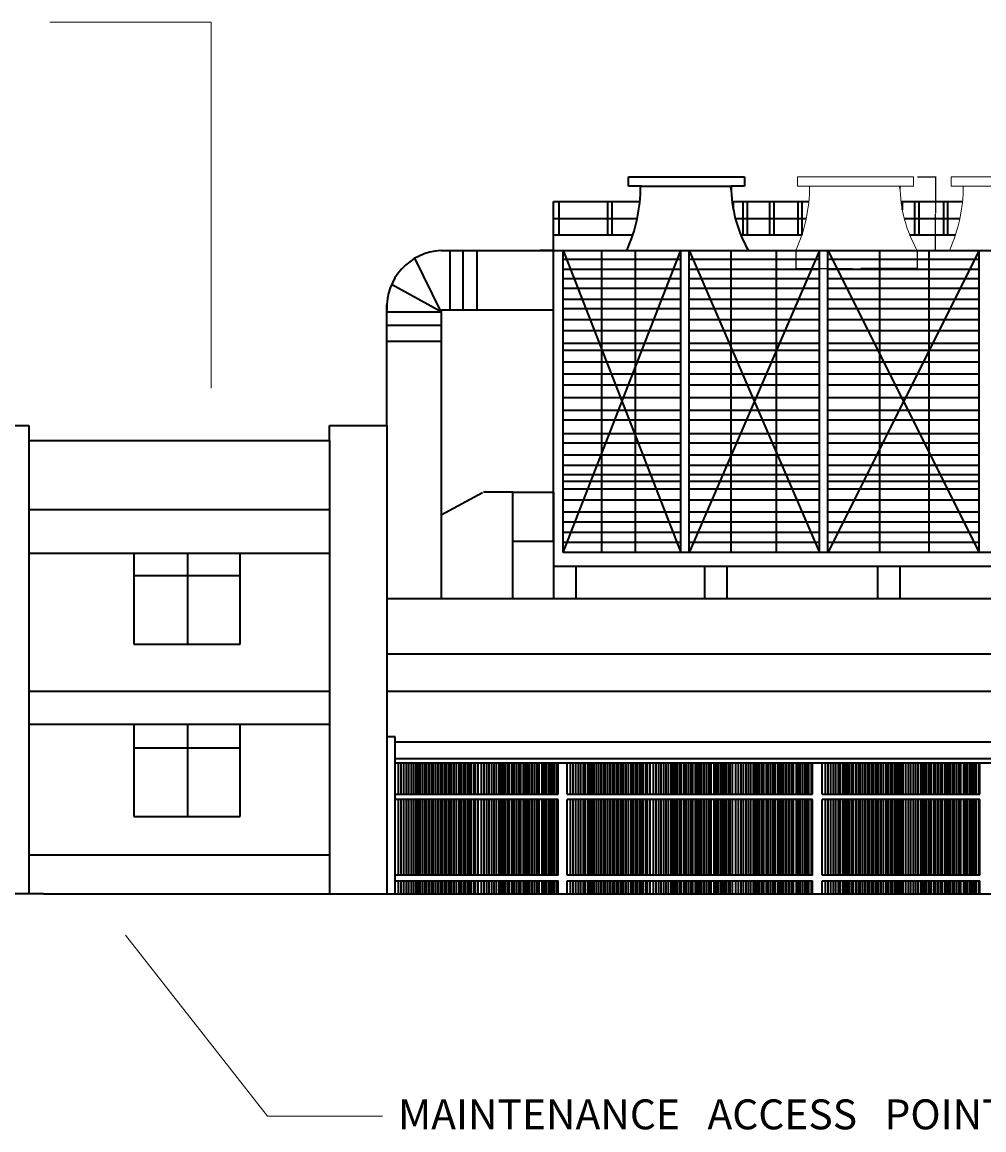
# Model space of a CAD drawing. Units: inches. Extents: x -1080 to 1950, y -1929 to 857.
# Tile 8 of 16: x 991 to 1333, y -819 to -424. Entities that reach past the tile are written whole.
import ezdxf

# ---------------------------------------------------------------- set-up
doc = ezdxf.new("R2010")
doc.units = ezdxf.units.IN
doc.header["$MEASUREMENT"] = 0
for name, color, linetype, lineweight in [('A-ANNO-DIMS', 2, 'Continuous', 18), ('A-ANNO-SYMB', 2, 'Continuous', 18), ('A-ANNO-TEXT', 7, 'Continuous', 25), ('A-DOOR', 3, 'Continuous', 18), ('A-ELEV', 7, 'Continuous', 35)]:
    doc.layers.add(name, color=color, linetype=linetype, lineweight=lineweight)
doc.styles.get("Standard").update_dxf_attribs({"font": 'arial.ttf'})
doc.dimstyles.get("Standard").update_dxf_attribs({"dimtxt": 0.18, "dimasz": 0.18, "dimexe": 0.18, "dimexo": 0.0625, "dimgap": 0.09, "dimtad": 0, "dimtih": 1, "dimtoh": 1, "dimdec": 4, "dimzin": 0, "dimdsep": 46, "dimtxsty": 'Standard', "dimcen": 0.09, "dimadec": 0, "dimazin": 0, "dimtfac": 1, "dimtdec": 4, "dimtofl": 0, "dimtmove": 0, "dimatfit": 3, "dimfxl": 1, "dimtolj": 1, "dimtzin": 0, "dimarcsym": 0})

# ---------------------------------------------------------------- blocks, each defined once
blk = doc.blocks.new('DOOR-DOUBLE')
for p, q in [((0.57, 22.87), (0.57, 26.22)), ((0.57, 26.22), (41.91, 26.22)), ((41.91, 26.22), (41.91, 22.87)), ((5.34, 22.87), (0.57, 22.87)), ((5.34, 22.87), (37.21, 22.87)), ((36.82, 22.87), (37.23, 21.43)), ((41.91, 22.87), (37.21, 22.87)), ((0, 0), (43.32, 0))]:
    blk.add_line(p, q)
for centre, radius, start, end in [((-50.66, 22.94), 55.61, 335.64, 359.9307), ((83.27, 22.93), 46.06, 180.0717, 209.8526)]:
    blk.add_arc(centre, radius, start, end)
blk = doc.blocks.new('*D79')
at = {"layer": 'A-ANNO-DIMS', "color": 0, "lineweight": -2, "transparency": 16777216}
for p, q in [((1266.17, -505.41), (1266.17, -512.02)), ((1309.49, -505.41), (1309.49, -512.02)), ((1266.35, -511.84), (1286.34, -511.84)), ((1309.31, -511.84), (1289.32, -511.84))]:
    blk.add_line(p, q, dxfattribs=at)
at = {"layer": 'A-ANNO-DIMS', "color": 0, "transparency": 16777216}
for points in [[(1266.35, -511.81), (1266.35, -511.87), (1266.17, -511.84)], [(1309.31, -511.81), (1309.31, -511.87), (1309.49, -511.84)]]:
    blk.add_solid(points, dxfattribs=at)
at = {"layer": 'Defpoints', "color": 0, "transparency": 16777216}
for p in [(1266.17, -505.35), (1309.49, -505.35), (1309.49, -511.84)]:
    blk.add_point(p, dxfattribs=at)
at = {"layer": 'A-ANNO-DIMS', "color": 0, "transparency": 16777216, "insert": (1287.83, -511.84), "char_height": 0.18, "attachment_point": 5}
blk.add_mtext('\\A1;DOUBLE DOOR 43 TYP.', dxfattribs=at)
blk = doc.blocks.new('*D80')
at = {"layer": 'A-ANNO-DIMS', "color": 0, "lineweight": -2, "transparency": 16777216}
for p, q in [((1309.55, -479.13), (1316.17, -479.13)), ((1315.99, -479.31), (1315.99, -492.06)), ((1315.99, -505.17), (1315.99, -492.42)), ((1309.55, -505.35), (1316.17, -505.35))]:
    blk.add_line(p, q, dxfattribs=at)
at = {"layer": 'A-ANNO-DIMS', "color": 0, "transparency": 16777216}
for points in [[(1315.96, -479.31), (1316.02, -479.31), (1315.99, -479.13)], [(1315.96, -505.17), (1316.02, -505.17), (1315.99, -505.35)]]:
    blk.add_solid(points, dxfattribs=at)
at = {"layer": 'Defpoints', "color": 0, "transparency": 16777216}
for p in [(1309.49, -479.13), (1315.99, -479.13), (1309.49, -505.35)]:
    blk.add_point(p, dxfattribs=at)
at = {"layer": 'A-ANNO-DIMS', "color": 0, "transparency": 16777216, "insert": (1315.99, -492.24), "char_height": 0.18, "attachment_point": 5}
blk.add_mtext('\\A1;26 TYP.', dxfattribs=at)

msp = doc.modelspace()

# ---------------------------------------------------------------- linework, layer by layer
at = {"layer": 'A-ANNO-SYMB'}
for p, q in [((1057.91, -423.98), (1000.41, -423.98)), ((1057.91, -554.48), (1057.91, -423.98)), ((1027.41, -749.48), (1077.91, -813.98)), ((1077.91, -813.98), (1118.91, -813.98))]:
    msp.add_line(p, q, dxfattribs=at)
at = {"layer": 'A-ELEV'}
for p, q in [((1206.53, -482.48), (1206.53, -479.13)), ((1206.53, -479.13), (1247.87, -479.13)), ((1247.87, -479.13), (1247.87, -482.48)), ((1211.3, -482.48), (1206.53, -482.48)), ((1211.3, -482.48), (1243.17, -482.48)), ((1242.79, -482.48), (1243.2, -483.92)), ((1247.87, -482.48), (1243.17, -482.48)), ((1179.83, -608.99), (1179.83, -487.89)), ((1179.83, -487.89), (1210.64, -487.89)), ((1179.83, -499.75), (1179.83, -487.89)), ((1179.83, -499.75), (1179.83, -487.89)), ((1181.87, -499.75), (1181.87, -487.89)), ((1199.22, -499.75), (1199.22, -487.89)), ((1200.79, -499.75), (1200.79, -487.89)), ((1243.5, -487.89), (1270.85, -487.89)), ((1243.96, -490.88), (1243.96, -487.89)), ((1247.41, -499.75), (1247.41, -487.89)), ((1248.98, -499.75), (1248.98, -487.89)), ((1256.91, -499.75), (1256.91, -487.89)), ((1258.48, -499.75), (1258.48, -487.89)), ((1267.07, -499.75), (1267.07, -487.89)), ((1268.4, -499.75), (1268.4, -487.89)), ((1303.71, -487.89), (1325.6, -487.89)), ((1304.16, -490.88), (1304.16, -487.89)), ((1308.56, -499.75), (1308.56, -487.89)), ((1310.13, -499.75), (1310.13, -487.89)), ((1318.88, -499.75), (1318.88, -487.89)), ((1320.33, -499.75), (1320.33, -487.89)), ((1179.83, -493.99), (1209.69, -493.99)), ((1244.65, -493.99), (1269.9, -493.99)), ((1304.86, -493.99), (1324.65, -493.99)), ((1179.83, -499.75), (1208.14, -499.75)), ((1246.56, -499.75), (1268.4, -499.75)), ((1306.76, -499.75), (1323.1, -499.75)), ((1139.81, -505.38), (1175.11, -505.38)), ((1142.91, -505.38), (1142.91, -526.67)), ((1147.55, -505.38), (1147.55, -526.67)), ((1152.58, -505.38), (1152.58, -526.67)), ((1179.83, -505.38), (1175.11, -505.38)), ((1175.11, -505.38), (1179.83, -505.38)), ((1179.83, -526.67), (1179.83, -505.38)), ((1179.83, -505.38), (1392.19, -505.38)), ((1183.24, -613.11), (1183.24, -505.38)), ((1183.24, -505.38), (1225.18, -505.38)), ((1183.24, -505.38), (1225.18, -613.11)), ((1183.24, -613.11), (1225.18, -505.38)), ((1197.1, -613.11), (1197.1, -505.38)), ((1205.96, -505.35), (1249.28, -505.35)), ((1209.07, -613.11), (1209.07, -505.38)), ((1225.18, -613.11), (1225.18, -505.38)), ((1228.25, -613.11), (1228.25, -505.38)), ((1228.25, -505.38), (1274.58, -613.11)), ((1274.58, -505.38), (1228.25, -613.11)), ((1228.25, -505.38), (1274.58, -505.38)), ((1243.17, -613.11), (1243.17, -505.38)), ((1259.32, -613.11), (1259.32, -505.38)), ((1274.58, -613.11), (1274.58, -505.38)), ((1277.65, -613.11), (1277.65, -505.38)), ((1277.65, -505.38), (1331.51, -613.11)), ((1331.51, -505.38), (1277.65, -613.11)), ((1277.65, -505.38), (1331.51, -505.38)), ((1296.11, -613.11), (1296.11, -505.38)), ((1313.76, -613.11), (1313.76, -505.38)), ((1331.51, -613.11), (1331.51, -505.38)), ((1139.81, -527.27), (1130.49, -508.15)), ((1183.24, -508.47), (1225.18, -508.47)), ((1228.25, -508.47), (1274.58, -508.47)), ((1277.65, -508.47), (1331.51, -508.47)), ((1183.24, -512.1), (1225.18, -512.1)), ((1228.25, -512.1), (1274.58, -512.1)), ((1277.65, -512.1), (1331.51, -512.1)), ((1183.24, -515.43), (1225.18, -515.43)), ((1228.25, -515.43), (1274.58, -515.43)), ((1277.65, -515.43), (1331.51, -515.43)), ((1139.81, -527.27), (1122.13, -517.55)), ((1183.24, -518.77), (1225.18, -518.77)), ((1228.25, -518.77), (1274.58, -518.77)), ((1277.65, -518.77), (1331.51, -518.77)), ((1120.45, -567.84), (1120.45, -524.75)), ((1183.24, -522.7), (1225.18, -522.7)), ((1228.25, -522.7), (1274.58, -522.7)), ((1277.65, -522.7), (1331.51, -522.7)), ((1120.45, -527.27), (1139.81, -527.27)), ((1175.11, -526.67), (1139.81, -526.67)), ((1139.81, -526.67), (1139.81, -629.59)), ((1179.83, -526.67), (1175.11, -526.67)), ((1183.24, -526.03), (1225.18, -526.03)), ((1228.25, -526.03), (1274.58, -526.03)), ((1277.65, -526.03), (1331.51, -526.03)), ((1120.45, -532.03), (1139.81, -532.03)), ((1183.24, -529.97), (1225.18, -529.97)), ((1228.25, -529.97), (1274.58, -529.97)), ((1277.65, -529.97), (1331.51, -529.97)), ((1183.24, -533.91), (1225.18, -533.91)), ((1228.25, -533.91), (1274.58, -533.91)), ((1277.65, -533.91), (1331.51, -533.91)), ((1120.45, -537.66), (1139.81, -537.66)), ((1129.33, -537.66), (1139.81, -537.66)), ((1130.5, -537.66), (1139.81, -537.66)), ((1130.83, -537.66), (1139.81, -537.66)), ((1183.24, -538.45), (1225.18, -538.45)), ((1183.24, -540.87), (1225.18, -540.87)), ((1228.25, -538.45), (1274.58, -538.45)), ((1228.25, -540.87), (1274.58, -540.87)), ((1277.65, -538.45), (1331.51, -538.45)), ((1277.65, -540.87), (1331.51, -540.87)), ((1183.24, -545.11), (1225.18, -545.11)), ((1228.25, -545.11), (1274.58, -545.11)), ((1277.65, -545.11), (1331.51, -545.11)), ((1183.24, -549.35), (1225.18, -549.35)), ((1228.25, -549.35), (1274.58, -549.35)), ((1277.65, -549.35), (1331.51, -549.35)), ((1183.24, -553.29), (1225.18, -553.29)), ((1228.25, -553.29), (1274.58, -553.29)), ((1277.65, -553.29), (1331.51, -553.29)), ((1183.24, -557.83), (1225.18, -557.83)), ((1228.25, -557.83), (1274.58, -557.83)), ((1277.65, -557.83), (1331.51, -557.83)), ((1183.24, -562.37), (1225.18, -562.37)), ((1228.25, -562.37), (1274.58, -562.37)), ((1277.65, -562.37), (1331.51, -562.37)), ((972.97, -567.84), (992.89, -567.84)), ((992.89, -567.84), (992.89, -734.72)), ((1099.99, -573.17), (1099.99, -567.84)), ((1099.99, -567.84), (1120.45, -567.84)), ((1120.45, -567.84), (1120.45, -734.72)), ((1183.24, -565.82), (1225.18, -565.82)), ((1228.25, -565.82), (1274.58, -565.82)), ((1277.65, -565.82), (1331.51, -565.82)), ((1183.24, -570.67), (1225.18, -570.67)), ((1228.25, -570.67), (1274.58, -570.67)), ((1277.65, -570.67), (1331.51, -570.67)), ((992.89, -573.17), (1099.99, -573.17)), ((1099.99, -573.17), (1099.99, -734.72)), ((1183.24, -574), (1225.18, -574)), ((1228.25, -574), (1274.58, -574)), ((1277.65, -574), (1331.51, -574)), ((1183.24, -578.24), (1225.18, -578.24)), ((1228.25, -578.24), (1274.58, -578.24)), ((1277.65, -578.24), (1331.51, -578.24)), ((1183.24, -581.87), (1225.18, -581.87)), ((1228.25, -581.87), (1274.58, -581.87)), ((1277.65, -581.87), (1331.51, -581.87)), ((1183.24, -585.21), (1225.18, -585.21)), ((1183.24, -587.63), (1225.18, -587.63)), ((1228.25, -585.21), (1274.58, -585.21)), ((1228.25, -587.63), (1274.58, -587.63)), ((1277.65, -585.21), (1331.51, -585.21)), ((1277.65, -587.63), (1331.51, -587.63)), ((1154.61, -591.76), (1139.81, -599.72)), ((1165.42, -591.58), (1154.87, -591.58)), ((1165.42, -629.59), (1165.42, -591.58)), ((1165.42, -591.58), (1179.83, -591.58)), ((1179.83, -591.58), (1179.83, -608.99)), ((1183.24, -590.35), (1225.18, -590.35)), ((1228.25, -590.35), (1274.58, -590.35)), ((1277.65, -590.35), (1331.51, -590.35)), ((1183.24, -594.29), (1225.18, -594.29)), ((1228.25, -594.29), (1274.58, -594.29)), ((1277.65, -594.29), (1331.51, -594.29)), ((992.89, -597.78), (1099.99, -597.78)), ((1183.24, -598.53), (1225.18, -598.53)), ((1228.25, -598.53), (1274.58, -598.53)), ((1277.65, -598.53), (1331.51, -598.53)), ((1183.24, -602.16), (1225.18, -602.16)), ((1228.25, -602.16), (1274.58, -602.16)), ((1277.65, -602.16), (1331.51, -602.16)), ((1183.24, -605.8), (1225.18, -605.8)), ((1228.25, -605.8), (1274.58, -605.8)), ((1277.65, -605.8), (1331.51, -605.8)), ((1165.42, -608.99), (1179.83, -608.99)), ((1179.83, -608.99), (1179.83, -629.59)), ((1183.24, -609.43), (1225.18, -609.43)), ((1228.25, -609.43), (1274.58, -609.43)), ((1277.65, -609.43), (1331.51, -609.43)), ((992.89, -613.27), (1099.99, -613.27)), ((1030.27, -613.27), (1030.27, -645.71)), ((1049.49, -613.27), (1049.49, -645.71)), ((1068.26, -645.71), (1068.26, -613.27)), ((1386.54, -613.11), (1183.24, -613.11)), ((1179.83, -617.91), (1392.19, -617.91)), ((1187.77, -617.91), (1187.77, -629.59)), ((1233.65, -617.91), (1233.65, -629.59)), ((1241.59, -617.91), (1241.59, -629.59)), ((1295.26, -617.91), (1295.26, -629.59)), ((1303.2, -617.91), (1303.2, -629.59)), ((1030.27, -621.22), (1068.26, -621.22)), ((1458.07, -629.59), (1120.45, -629.59)), ((1030.27, -645.71), (1068.26, -645.71)), ((1458.07, -649.29), (1120.45, -649.29)), ((992.89, -662.56), (1099.99, -662.56)), ((1120.45, -662.56), (1458.07, -662.56)), ((992.89, -674.3), (1099.99, -674.3)), ((1030.27, -674.75), (1030.27, -707.19)), ((1049.49, -674.75), (1049.49, -707.19)), ((1068.26, -707.19), (1068.26, -674.75)), ((1123.47, -678.74), (1120.45, -678.74)), ((1123.47, -688.04), (1123.47, -678.74)), ((1030.27, -682.7), (1068.26, -682.7)), ((1627.86, -680.68), (1123.47, -680.68)), ((1123.47, -686.45), (1622.49, -686.45)), ((1123.47, -688.04), (1622.49, -688.04)), ((1123.47, -699.19), (1123.47, -688.04)), ((1123.47, -688.04), (1123.47, -688.04)), ((1124.66, -699.19), (1124.66, -688.04)), ((1125.63, -699.19), (1125.63, -688.04)), ((1126.55, -699.19), (1126.55, -688.04)), ((1127.44, -699.19), (1127.44, -688.04)), ((1128.36, -699.19), (1128.36, -688.04)), ((1129.24, -699.19), (1129.24, -688.04)), ((1130.03, -699.19), (1130.03, -688.04)), ((1130.96, -699.19), (1130.96, -688.04)), ((1131.66, -699.19), (1131.66, -688.04)), ((1132.37, -699.19), (1132.37, -688.04)), ((1133.12, -699.19), (1133.12, -688.04)), ((1133.95, -699.19), (1133.95, -688.04)), ((1134.67, -699.19), (1134.67, -688.04)), ((1135.57, -699.19), (1135.57, -688.04)), ((1136.36, -699.19), (1136.36, -688.04)), ((1137.15, -699.19), (1137.15, -688.04)), ((1137.94, -699.19), (1137.94, -688.04)), ((1138.73, -699.19), (1138.73, -688.04)), ((1139.63, -699.19), (1139.63, -688.04)), ((1140.3, -699.19), (1140.3, -688.04)), ((1141.09, -699.19), (1141.09, -688.04)), ((1141.66, -699.19), (1141.66, -688.04)), ((1142.44, -699.19), (1142.44, -688.04)), ((1142.9, -699.19), (1142.9, -688.04)), ((1143.68, -699.19), (1143.68, -688.04)), ((1144.47, -699.19), (1144.47, -688.04)), ((1145.26, -699.19), (1145.26, -688.04)), ((1146.28, -699.19), (1146.28, -688.04)), ((1146.95, -699.19), (1146.95, -688.04)), ((1147.74, -699.19), (1147.74, -688.04)), ((1148.53, -699.19), (1148.53, -688.04)), ((1149.32, -699.19), (1149.32, -688.04)), ((1150, -699.19), (1150, -688.04)), ((1150.67, -699.19), (1150.67, -688.04)), ((1151.57, -699.19), (1151.57, -688.04)), ((1152.03, -699.19), (1152.03, -688.04)), ((1152.99, -699.19), (1152.99, -688.04)), ((1154.18, -699.19), (1154.18, -688.04)), ((1155.15, -699.19), (1155.15, -688.04)), ((1156.08, -699.19), (1156.08, -688.04)), ((1156.96, -699.19), (1156.96, -688.04)), ((1157.88, -699.19), (1157.88, -688.04)), ((1158.76, -699.19), (1158.76, -688.04)), ((1159.56, -699.19), (1159.56, -688.04)), ((1160.48, -699.19), (1160.48, -688.04)), ((1161.19, -699.19), (1161.19, -688.04)), ((1161.89, -699.19), (1161.89, -688.04)), ((1162.64, -699.19), (1162.64, -688.04)), ((1163.48, -699.19), (1163.48, -688.04)), ((1164.19, -699.19), (1164.19, -688.04)), ((1165.09, -699.19), (1165.09, -688.04)), ((1165.88, -699.19), (1165.88, -688.04)), ((1166.67, -699.19), (1166.67, -688.04)), ((1167.46, -699.19), (1167.46, -688.04)), ((1168.25, -699.19), (1168.25, -688.04)), ((1169.15, -699.19), (1169.15, -688.04)), ((1169.83, -699.19), (1169.83, -688.04)), ((1170.61, -699.19), (1170.61, -688.04)), ((1171.18, -699.19), (1171.18, -688.04)), ((1171.97, -699.19), (1171.97, -688.04)), ((1172.42, -699.19), (1172.42, -688.04)), ((1173.21, -699.19), (1173.21, -688.04)), ((1174, -699.19), (1174, -688.04)), ((1174.79, -699.19), (1174.79, -688.04)), ((1175.8, -699.19), (1175.8, -688.04)), ((1176.48, -699.19), (1176.48, -688.04)), ((1177.27, -699.19), (1177.27, -688.04)), ((1178.05, -699.19), (1178.05, -688.04)), ((1178.84, -699.19), (1178.84, -688.04)), ((1179.52, -699.19), (1179.52, -688.04)), ((1180.2, -699.19), (1180.2, -688.04)), ((1181.1, -699.19), (1181.1, -688.04)), ((1181.55, -699.19), (1181.55, -688.04)), ((1184.75, -699.19), (1184.75, -688.04)), ((1185.94, -699.19), (1185.94, -688.04)), ((1186.91, -699.19), (1186.91, -688.04)), ((1187.83, -699.19), (1187.83, -688.04)), ((1188.71, -699.19), (1188.71, -688.04)), ((1189.64, -699.19), (1189.64, -688.04)), ((1190.52, -699.19), (1190.52, -688.04)), ((1191.31, -699.19), (1191.31, -688.04)), ((1192.24, -699.19), (1192.24, -688.04)), ((1192.94, -699.19), (1192.94, -688.04)), ((1193.65, -699.19), (1193.65, -688.04)), ((1194.4, -699.19), (1194.4, -688.04)), ((1195.23, -699.19), (1195.23, -688.04)), ((1195.95, -699.19), (1195.95, -688.04)), ((1196.85, -699.19), (1196.85, -688.04)), ((1197.64, -699.19), (1197.64, -688.04)), ((1198.43, -699.19), (1198.43, -688.04)), ((1199.22, -699.19), (1199.22, -688.04)), ((1200, -699.19), (1200, -688.04)), ((1200.91, -699.19), (1200.91, -688.04)), ((1201.58, -699.19), (1201.58, -688.04)), ((1202.37, -699.19), (1202.37, -688.04)), ((1202.93, -699.19), (1202.93, -688.04)), ((1203.72, -699.19), (1203.72, -688.04)), ((1204.17, -699.19), (1204.17, -688.04)), ((1204.96, -699.19), (1204.96, -688.04)), ((1205.75, -699.19), (1205.75, -688.04)), ((1206.54, -699.19), (1206.54, -688.04)), ((1207.56, -699.19), (1207.56, -688.04)), ((1208.23, -699.19), (1208.23, -688.04)), ((1209.02, -699.19), (1209.02, -688.04)), ((1209.81, -699.19), (1209.81, -688.04)), ((1210.6, -699.19), (1210.6, -688.04)), ((1211.28, -699.19), (1211.28, -688.04)), ((1211.95, -699.19), (1211.95, -688.04)), ((1212.85, -699.19), (1212.85, -688.04)), ((1213.3, -699.19), (1213.3, -688.04)), ((1214.28, -699.19), (1214.28, -688.04)), ((1215.47, -699.19), (1215.47, -688.04)), ((1216.44, -699.19), (1216.44, -688.04)), ((1217.36, -699.19), (1217.36, -688.04)), ((1218.24, -699.19), (1218.24, -688.04)), ((1219.17, -699.19), (1219.17, -688.04)), ((1220.05, -699.19), (1220.05, -688.04)), ((1220.84, -699.19), (1220.84, -688.04)), ((1221.77, -699.19), (1221.77, -688.04)), ((1222.47, -699.19), (1222.47, -688.04)), ((1223.18, -699.19), (1223.18, -688.04)), ((1223.93, -699.19), (1223.93, -688.04)), ((1224.76, -699.19), (1224.76, -688.04)), ((1225.48, -699.19), (1225.48, -688.04)), ((1226.38, -699.19), (1226.38, -688.04)), ((1227.17, -699.19), (1227.17, -688.04)), ((1227.96, -699.19), (1227.96, -688.04)), ((1228.74, -699.19), (1228.74, -688.04)), ((1229.53, -699.19), (1229.53, -688.04)), ((1230.44, -699.19), (1230.44, -688.04)), ((1231.11, -699.19), (1231.11, -688.04)), ((1231.9, -699.19), (1231.9, -688.04)), ((1232.46, -699.19), (1232.46, -688.04)), ((1233.25, -699.19), (1233.25, -688.04)), ((1233.7, -699.19), (1233.7, -688.04)), ((1234.49, -699.19), (1234.49, -688.04)), ((1235.28, -699.19), (1235.28, -688.04)), ((1236.07, -699.19), (1236.07, -688.04)), ((1237.09, -699.19), (1237.09, -688.04)), ((1237.76, -699.19), (1237.76, -688.04)), ((1238.55, -699.19), (1238.55, -688.04)), ((1239.34, -699.19), (1239.34, -688.04)), ((1240.13, -699.19), (1240.13, -688.04)), ((1240.81, -699.19), (1240.81, -688.04)), ((1241.48, -699.19), (1241.48, -688.04)), ((1242.38, -699.19), (1242.38, -688.04)), ((1242.83, -699.19), (1242.83, -688.04)), ((1243.62, -699.19), (1243.62, -688.04)), ((1244.81, -699.19), (1244.81, -688.04)), ((1245.78, -699.19), (1245.78, -688.04)), ((1246.71, -699.19), (1246.71, -688.04)), ((1247.59, -699.19), (1247.59, -688.04)), ((1248.51, -699.19), (1248.51, -688.04)), ((1249.39, -699.19), (1249.39, -688.04)), ((1250.19, -699.19), (1250.19, -688.04)), ((1251.11, -699.19), (1251.11, -688.04)), ((1251.82, -699.19), (1251.82, -688.04)), ((1252.52, -699.19), (1252.52, -688.04)), ((1253.27, -699.19), (1253.27, -688.04)), ((1254.11, -699.19), (1254.11, -688.04)), ((1254.82, -699.19), (1254.82, -688.04)), ((1255.72, -699.19), (1255.72, -688.04)), ((1256.51, -699.19), (1256.51, -688.04)), ((1257.3, -699.19), (1257.3, -688.04)), ((1258.09, -699.19), (1258.09, -688.04)), ((1258.88, -699.19), (1258.88, -688.04)), ((1259.78, -699.19), (1259.78, -688.04)), ((1260.46, -699.19), (1260.46, -688.04)), ((1261.24, -699.19), (1261.24, -688.04)), ((1261.81, -699.19), (1261.81, -688.04)), ((1262.6, -699.19), (1262.6, -688.04)), ((1263.05, -699.19), (1263.05, -688.04)), ((1263.84, -699.19), (1263.84, -688.04)), ((1264.63, -699.19), (1264.63, -688.04)), ((1265.41, -699.19), (1265.41, -688.04)), ((1266.43, -699.19), (1266.43, -688.04)), ((1267.11, -699.19), (1267.11, -688.04)), ((1267.89, -699.19), (1267.89, -688.04)), ((1268.68, -699.19), (1268.68, -688.04)), ((1269.47, -699.19), (1269.47, -688.04)), ((1270.15, -699.19), (1270.15, -688.04)), ((1270.83, -699.19), (1270.83, -688.04)), ((1271.73, -699.19), (1271.73, -688.04)), ((1272.18, -699.19), (1272.18, -688.04)), ((1275.6, -699.19), (1275.6, -688.04)), ((1276.8, -699.19), (1276.8, -688.04)), ((1277.77, -699.19), (1277.77, -688.04)), ((1278.69, -699.19), (1278.69, -688.04)), ((1279.57, -699.19), (1279.57, -688.04)), ((1280.5, -699.19), (1280.5, -688.04)), ((1281.38, -699.19), (1281.38, -688.04)), ((1282.17, -699.19), (1282.17, -688.04)), ((1283.1, -699.19), (1283.1, -688.04)), ((1283.8, -699.19), (1283.8, -688.04)), ((1284.5, -699.19), (1284.5, -688.04)), ((1285.25, -699.19), (1285.25, -688.04)), ((1286.09, -699.19), (1286.09, -688.04)), ((1286.8, -699.19), (1286.8, -688.04)), ((1287.71, -699.19), (1287.71, -688.04)), ((1288.49, -699.19), (1288.49, -688.04)), ((1289.28, -699.19), (1289.28, -688.04)), ((1290.07, -699.19), (1290.07, -688.04)), ((1290.86, -699.19), (1290.86, -688.04)), ((1291.76, -699.19), (1291.76, -688.04)), ((1292.44, -699.19), (1292.44, -688.04)), ((1293.23, -699.19), (1293.23, -688.04)), ((1293.79, -699.19), (1293.79, -688.04)), ((1294.58, -699.19), (1294.58, -688.04)), ((1295.03, -699.19), (1295.03, -688.04)), ((1295.82, -699.19), (1295.82, -688.04)), ((1296.61, -699.19), (1296.61, -688.04)), ((1297.4, -699.19), (1297.4, -688.04)), ((1298.41, -699.19), (1298.41, -688.04)), ((1299.09, -699.19), (1299.09, -688.04)), ((1299.88, -699.19), (1299.88, -688.04)), ((1300.67, -699.19), (1300.67, -688.04)), ((1301.46, -699.19), (1301.46, -688.04)), ((1302.13, -699.19), (1302.13, -688.04)), ((1302.81, -699.19), (1302.81, -688.04)), ((1303.24, -699.19), (1303.24, -688.04)), ((1303.71, -699.19), (1303.71, -688.04)), ((1304.16, -699.19), (1304.16, -688.04)), ((1304.43, -699.19), (1304.43, -688.04)), ((1305.4, -699.19), (1305.4, -688.04)), ((1306.33, -699.19), (1306.33, -688.04)), ((1307.21, -699.19), (1307.21, -688.04)), ((1308.13, -699.19), (1308.13, -688.04)), ((1309.01, -699.19), (1309.01, -688.04)), ((1309.81, -699.19), (1309.81, -688.04)), ((1310.73, -699.19), (1310.73, -688.04)), ((1311.44, -699.19), (1311.44, -688.04)), ((1312.14, -699.19), (1312.14, -688.04)), ((1312.89, -699.19), (1312.89, -688.04)), ((1313.73, -699.19), (1313.73, -688.04)), ((1314.44, -699.19), (1314.44, -688.04)), ((1315.34, -699.19), (1315.34, -688.04)), ((1316.13, -699.19), (1316.13, -688.04)), ((1316.92, -699.19), (1316.92, -688.04)), ((1317.71, -699.19), (1317.71, -688.04)), ((1318.5, -699.19), (1318.5, -688.04)), ((1319.4, -699.19), (1319.4, -688.04)), ((1320.08, -699.19), (1320.08, -688.04)), ((1320.87, -699.19), (1320.87, -688.04)), ((1321.43, -699.19), (1321.43, -688.04)), ((1322.22, -699.19), (1322.22, -688.04)), ((1322.67, -699.19), (1322.67, -688.04)), ((1323.46, -699.19), (1323.46, -688.04)), ((1324.25, -699.19), (1324.25, -688.04)), ((1325.04, -699.19), (1325.04, -688.04)), ((1326.05, -699.19), (1326.05, -688.04)), ((1326.73, -699.19), (1326.73, -688.04)), ((1327.52, -699.19), (1327.52, -688.04)), ((1328.3, -699.19), (1328.3, -688.04)), ((1329.09, -699.19), (1329.09, -688.04)), ((1329.77, -699.19), (1329.77, -688.04)), ((1330.45, -699.19), (1330.45, -688.04)), ((1331.35, -699.19), (1331.35, -688.04)), ((1331.8, -699.19), (1331.8, -688.04)), ((1123.47, -728.07), (1123.47, -699.19)), ((1123.47, -699.19), (1181.55, -699.19)), ((1181.55, -701.07), (1123.47, -701.07)), ((1124.66, -728.07), (1124.66, -701.07)), ((1125.63, -728.07), (1125.63, -701.07)), ((1126.55, -728.07), (1126.55, -701.07)), ((1127.44, -728.07), (1127.44, -701.07)), ((1128.36, -728.07), (1128.36, -701.07)), ((1129.24, -728.07), (1129.24, -701.07)), ((1130.03, -728.07), (1130.03, -701.07)), ((1130.96, -728.07), (1130.96, -701.07)), ((1131.66, -728.07), (1131.66, -701.07)), ((1132.37, -728.07), (1132.37, -701.07)), ((1133.12, -728.07), (1133.12, -701.07)), ((1133.95, -728.07), (1133.95, -701.07)), ((1134.67, -728.07), (1134.67, -701.07)), ((1135.57, -728.07), (1135.57, -701.07)), ((1136.36, -728.07), (1136.36, -701.07)), ((1137.15, -728.07), (1137.15, -701.07)), ((1137.94, -728.07), (1137.94, -701.07)), ((1138.73, -728.07), (1138.73, -701.07)), ((1139.63, -728.07), (1139.63, -701.07)), ((1140.3, -728.07), (1140.3, -701.07)), ((1141.09, -728.07), (1141.09, -701.07)), ((1141.66, -728.07), (1141.66, -701.07)), ((1142.44, -728.07), (1142.44, -701.07)), ((1142.9, -728.07), (1142.9, -701.07)), ((1143.68, -728.07), (1143.68, -701.07)), ((1144.47, -728.07), (1144.47, -701.07)), ((1145.26, -728.07), (1145.26, -701.07)), ((1146.28, -728.07), (1146.28, -701.07)), ((1146.95, -728.07), (1146.95, -701.07)), ((1147.74, -728.07), (1147.74, -701.07)), ((1148.53, -728.07), (1148.53, -701.07)), ((1149.32, -728.07), (1149.32, -701.07)), ((1150, -728.07), (1150, -701.07)), ((1150.67, -728.07), (1150.67, -701.07)), ((1151.57, -728.07), (1151.57, -701.07)), ((1152.03, -728.07), (1152.03, -701.07)), ((1152.99, -728.07), (1152.99, -701.07)), ((1154.18, -728.07), (1154.18, -701.07)), ((1155.15, -728.07), (1155.15, -701.07)), ((1156.08, -728.07), (1156.08, -701.07)), ((1156.96, -728.07), (1156.96, -701.07)), ((1157.88, -728.07), (1157.88, -701.07)), ((1158.76, -728.07), (1158.76, -701.07)), ((1159.56, -728.07), (1159.56, -701.07)), ((1160.48, -728.07), (1160.48, -701.07)), ((1161.19, -728.07), (1161.19, -701.07)), ((1161.89, -728.07), (1161.89, -701.07)), ((1162.64, -728.07), (1162.64, -701.07)), ((1163.48, -728.07), (1163.48, -701.07)), ((1164.19, -728.07), (1164.19, -701.07)), ((1165.09, -728.07), (1165.09, -701.07)), ((1165.88, -728.07), (1165.88, -701.07)), ((1166.67, -728.07), (1166.67, -701.07)), ((1167.46, -728.07), (1167.46, -701.07)), ((1168.25, -728.07), (1168.25, -701.07)), ((1169.15, -728.07), (1169.15, -701.07)), ((1169.83, -728.07), (1169.83, -701.07)), ((1170.61, -728.07), (1170.61, -701.07)), ((1171.18, -728.07), (1171.18, -701.07)), ((1171.97, -728.07), (1171.97, -701.07)), ((1172.42, -728.07), (1172.42, -701.07)), ((1173.21, -728.07), (1173.21, -701.07)), ((1174, -728.07), (1174, -701.07)), ((1174.79, -728.07), (1174.79, -701.07)), ((1175.8, -728.07), (1175.8, -701.07)), ((1176.48, -728.07), (1176.48, -701.07)), ((1177.27, -728.07), (1177.27, -701.07)), ((1178.05, -728.07), (1178.05, -701.07)), ((1178.84, -728.07), (1178.84, -701.07)), ((1179.52, -728.07), (1179.52, -701.07)), ((1180.2, -728.07), (1180.2, -701.07)), ((1181.1, -728.07), (1181.1, -701.07)), ((1181.55, -728.07), (1181.55, -701.07)), ((1184.75, -699.19), (1272.18, -699.19)), ((1184.75, -728.07), (1184.75, -701.07)), ((1272.18, -701.07), (1184.75, -701.07)), ((1185.94, -728.07), (1185.94, -701.07)), ((1186.91, -728.07), (1186.91, -701.07)), ((1187.83, -728.07), (1187.83, -701.07)), ((1188.71, -728.07), (1188.71, -701.07)), ((1189.64, -728.07), (1189.64, -701.07)), ((1190.52, -728.07), (1190.52, -701.07)), ((1191.31, -728.07), (1191.31, -701.07)), ((1192.24, -728.07), (1192.24, -701.07)), ((1192.94, -728.07), (1192.94, -701.07)), ((1193.65, -728.07), (1193.65, -701.07)), ((1194.4, -728.07), (1194.4, -701.07)), ((1195.23, -728.07), (1195.23, -701.07)), ((1195.95, -728.07), (1195.95, -701.07)), ((1196.85, -728.07), (1196.85, -701.07)), ((1197.64, -728.07), (1197.64, -701.07)), ((1198.43, -728.07), (1198.43, -701.07)), ((1199.22, -728.07), (1199.22, -701.07)), ((1200, -728.07), (1200, -701.07)), ((1200.91, -728.07), (1200.91, -701.07)), ((1201.58, -728.07), (1201.58, -701.07)), ((1202.37, -728.07), (1202.37, -701.07)), ((1202.93, -728.07), (1202.93, -701.07)), ((1203.72, -728.07), (1203.72, -701.07)), ((1204.17, -728.07), (1204.17, -701.07)), ((1204.96, -728.07), (1204.96, -701.07)), ((1205.75, -728.07), (1205.75, -701.07)), ((1206.54, -728.07), (1206.54, -701.07)), ((1207.56, -728.07), (1207.56, -701.07)), ((1208.23, -728.07), (1208.23, -701.07)), ((1209.02, -728.07), (1209.02, -701.07)), ((1209.81, -728.07), (1209.81, -701.07)), ((1210.6, -728.07), (1210.6, -701.07)), ((1211.28, -728.07), (1211.28, -701.07)), ((1211.95, -728.07), (1211.95, -701.07)), ((1212.85, -728.07), (1212.85, -701.07)), ((1213.3, -728.07), (1213.3, -701.07)), ((1214.28, -728.07), (1214.28, -701.07)), ((1215.47, -728.07), (1215.47, -701.07)), ((1216.44, -728.07), (1216.44, -701.07)), ((1217.36, -728.07), (1217.36, -701.07)), ((1218.24, -728.07), (1218.24, -701.07)), ((1219.17, -728.07), (1219.17, -701.07)), ((1220.05, -728.07), (1220.05, -701.07)), ((1220.84, -728.07), (1220.84, -701.07)), ((1221.77, -728.07), (1221.77, -701.07)), ((1222.47, -728.07), (1222.47, -701.07)), ((1223.18, -728.07), (1223.18, -701.07)), ((1223.93, -728.07), (1223.93, -701.07)), ((1224.76, -728.07), (1224.76, -701.07)), ((1225.48, -728.07), (1225.48, -701.07)), ((1226.38, -728.07), (1226.38, -701.07)), ((1227.17, -728.07), (1227.17, -701.07)), ((1227.96, -728.07), (1227.96, -701.07)), ((1228.74, -728.07), (1228.74, -701.07)), ((1229.53, -728.07), (1229.53, -701.07)), ((1230.44, -728.07), (1230.44, -701.07)), ((1231.11, -728.07), (1231.11, -701.07)), ((1231.9, -728.07), (1231.9, -701.07)), ((1232.46, -728.07), (1232.46, -701.07)), ((1233.25, -728.07), (1233.25, -701.07)), ((1233.7, -728.07), (1233.7, -701.07)), ((1234.49, -728.07), (1234.49, -701.07)), ((1235.28, -728.07), (1235.28, -701.07)), ((1236.07, -728.07), (1236.07, -701.07)), ((1237.09, -728.07), (1237.09, -701.07)), ((1237.76, -728.07), (1237.76, -701.07)), ((1238.55, -728.07), (1238.55, -701.07)), ((1239.34, -728.07), (1239.34, -701.07)), ((1240.13, -728.07), (1240.13, -701.07)), ((1240.81, -728.07), (1240.81, -701.07)), ((1241.48, -728.07), (1241.48, -701.07)), ((1242.38, -728.07), (1242.38, -701.07)), ((1242.83, -728.07), (1242.83, -701.07)), ((1243.62, -728.07), (1243.62, -701.07)), ((1244.81, -728.07), (1244.81, -701.07)), ((1245.78, -728.07), (1245.78, -701.07)), ((1246.71, -728.07), (1246.71, -701.07)), ((1247.59, -728.07), (1247.59, -701.07)), ((1248.51, -728.07), (1248.51, -701.07)), ((1249.39, -728.07), (1249.39, -701.07)), ((1250.19, -728.07), (1250.19, -701.07)), ((1251.11, -728.07), (1251.11, -701.07)), ((1251.82, -728.07), (1251.82, -701.07)), ((1252.52, -728.07), (1252.52, -701.07)), ((1253.27, -728.07), (1253.27, -701.07)), ((1254.11, -728.07), (1254.11, -701.07)), ((1254.82, -728.07), (1254.82, -701.07)), ((1255.72, -728.07), (1255.72, -701.07)), ((1256.51, -728.07), (1256.51, -701.07)), ((1257.3, -728.07), (1257.3, -701.07)), ((1258.09, -728.07), (1258.09, -701.07)), ((1258.88, -728.07), (1258.88, -701.07)), ((1259.78, -728.07), (1259.78, -701.07)), ((1260.46, -728.07), (1260.46, -701.07)), ((1261.24, -728.07), (1261.24, -701.07)), ((1261.81, -728.07), (1261.81, -701.07)), ((1262.6, -728.07), (1262.6, -701.07)), ((1263.05, -728.07), (1263.05, -701.07)), ((1263.84, -728.07), (1263.84, -701.07)), ((1264.63, -728.07), (1264.63, -701.07)), ((1265.41, -728.07), (1265.41, -701.07)), ((1266.43, -728.07), (1266.43, -701.07)), ((1267.11, -728.07), (1267.11, -701.07)), ((1267.89, -728.07), (1267.89, -701.07)), ((1268.68, -728.07), (1268.68, -701.07)), ((1269.47, -728.07), (1269.47, -701.07)), ((1270.15, -728.07), (1270.15, -701.07)), ((1270.83, -728.07), (1270.83, -701.07)), ((1271.73, -728.07), (1271.73, -701.07)), ((1272.18, -728.07), (1272.18, -701.07)), ((1275.6, -699.19), (1331.8, -699.19)), ((1275.6, -728.07), (1275.6, -701.07)), ((1331.8, -701.07), (1275.6, -701.07)), ((1276.8, -728.07), (1276.8, -701.07)), ((1277.77, -728.07), (1277.77, -701.07)), ((1278.69, -728.07), (1278.69, -701.07)), ((1279.57, -728.07), (1279.57, -701.07)), ((1280.5, -728.07), (1280.5, -701.07)), ((1281.38, -728.07), (1281.38, -701.07)), ((1282.17, -728.07), (1282.17, -701.07)), ((1283.1, -728.07), (1283.1, -701.07)), ((1283.8, -728.07), (1283.8, -701.07)), ((1284.5, -728.07), (1284.5, -701.07)), ((1285.25, -728.07), (1285.25, -701.07)), ((1286.09, -728.07), (1286.09, -701.07)), ((1286.8, -728.07), (1286.8, -701.07)), ((1287.71, -728.07), (1287.71, -701.07)), ((1288.49, -728.07), (1288.49, -701.07)), ((1289.28, -728.07), (1289.28, -701.07)), ((1290.07, -728.07), (1290.07, -701.07)), ((1290.86, -728.07), (1290.86, -701.07)), ((1291.76, -728.07), (1291.76, -701.07)), ((1292.44, -728.07), (1292.44, -701.07)), ((1293.23, -728.07), (1293.23, -701.07)), ((1293.79, -728.07), (1293.79, -701.07)), ((1294.58, -728.07), (1294.58, -701.07)), ((1295.03, -728.07), (1295.03, -701.07)), ((1295.82, -728.07), (1295.82, -701.07)), ((1296.61, -728.07), (1296.61, -701.07)), ((1297.4, -728.07), (1297.4, -701.07)), ((1298.41, -728.07), (1298.41, -701.07)), ((1299.09, -728.07), (1299.09, -701.07)), ((1299.88, -728.07), (1299.88, -701.07)), ((1300.67, -728.07), (1300.67, -701.07)), ((1301.46, -728.07), (1301.46, -701.07)), ((1302.13, -728.07), (1302.13, -701.07)), ((1302.81, -728.07), (1302.81, -701.07)), ((1303.24, -728.07), (1303.24, -701.07)), ((1303.71, -728.07), (1303.71, -701.07)), ((1304.16, -728.07), (1304.16, -701.07)), ((1304.43, -728.07), (1304.43, -701.07)), ((1305.4, -728.07), (1305.4, -701.07)), ((1306.33, -728.07), (1306.33, -701.07)), ((1307.21, -728.07), (1307.21, -701.07)), ((1308.13, -728.07), (1308.13, -701.07)), ((1309.01, -728.07), (1309.01, -701.07)), ((1309.81, -728.07), (1309.81, -701.07)), ((1310.73, -728.07), (1310.73, -701.07)), ((1311.44, -728.07), (1311.44, -701.07)), ((1312.14, -728.07), (1312.14, -701.07)), ((1312.89, -728.07), (1312.89, -701.07)), ((1313.73, -728.07), (1313.73, -701.07)), ((1314.44, -728.07), (1314.44, -701.07)), ((1315.34, -728.07), (1315.34, -701.07)), ((1316.13, -728.07), (1316.13, -701.07)), ((1316.92, -728.07), (1316.92, -701.07)), ((1317.71, -728.07), (1317.71, -701.07)), ((1318.5, -728.07), (1318.5, -701.07)), ((1319.4, -728.07), (1319.4, -701.07)), ((1320.08, -728.07), (1320.08, -701.07)), ((1320.87, -728.07), (1320.87, -701.07)), ((1321.43, -728.07), (1321.43, -701.07)), ((1322.22, -728.07), (1322.22, -701.07)), ((1322.67, -728.07), (1322.67, -701.07)), ((1323.46, -728.07), (1323.46, -701.07)), ((1324.25, -728.07), (1324.25, -701.07)), ((1325.04, -728.07), (1325.04, -701.07)), ((1326.05, -728.07), (1326.05, -701.07)), ((1326.73, -728.07), (1326.73, -701.07)), ((1327.52, -728.07), (1327.52, -701.07)), ((1328.3, -728.07), (1328.3, -701.07)), ((1329.09, -728.07), (1329.09, -701.07)), ((1329.77, -728.07), (1329.77, -701.07)), ((1330.45, -728.07), (1330.45, -701.07)), ((1331.35, -728.07), (1331.35, -701.07)), ((1331.8, -728.07), (1331.8, -701.07)), ((1030.27, -707.19), (1068.26, -707.19)), ((992.89, -720.85), (1099.99, -720.85)), ((1123.47, -734.72), (1123.47, -728.07)), ((1181.55, -728.07), (1123.47, -728.07)), ((1123.47, -730.16), (1181.55, -730.16)), ((1124.66, -734.72), (1124.66, -730.16)), ((1125.63, -734.72), (1125.63, -730.16)), ((1126.55, -734.72), (1126.55, -730.16)), ((1127.44, -734.72), (1127.44, -730.16)), ((1128.36, -734.72), (1128.36, -730.16)), ((1129.24, -734.72), (1129.24, -730.16)), ((1130.03, -734.72), (1130.03, -730.16)), ((1130.96, -734.72), (1130.96, -730.16)), ((1131.66, -734.72), (1131.66, -730.16)), ((1132.37, -734.72), (1132.37, -730.16)), ((1133.12, -734.72), (1133.12, -730.16)), ((1133.95, -734.72), (1133.95, -730.16)), ((1134.67, -734.72), (1134.67, -730.16)), ((1135.57, -734.72), (1135.57, -730.16)), ((1136.36, -734.72), (1136.36, -730.16)), ((1137.15, -734.72), (1137.15, -730.16)), ((1137.94, -734.72), (1137.94, -730.16)), ((1138.73, -734.72), (1138.73, -730.16)), ((1139.63, -734.72), (1139.63, -730.16)), ((1140.3, -734.72), (1140.3, -730.16)), ((1141.09, -734.72), (1141.09, -730.16)), ((1141.66, -734.72), (1141.66, -730.16)), ((1142.44, -734.72), (1142.44, -730.16)), ((1142.9, -734.72), (1142.9, -730.16)), ((1143.68, -734.72), (1143.68, -730.16)), ((1144.47, -734.72), (1144.47, -730.16)), ((1145.26, -734.72), (1145.26, -730.16)), ((1146.28, -734.72), (1146.28, -730.16)), ((1146.95, -734.72), (1146.95, -730.16)), ((1147.74, -734.72), (1147.74, -730.16)), ((1148.53, -734.72), (1148.53, -730.16)), ((1149.32, -734.72), (1149.32, -730.16)), ((1150, -734.72), (1150, -730.16)), ((1150.67, -734.72), (1150.67, -730.16)), ((1151.57, -734.72), (1151.57, -730.16)), ((1152.03, -734.72), (1152.03, -730.16)), ((1152.99, -734.72), (1152.99, -730.16)), ((1154.18, -734.72), (1154.18, -730.16)), ((1155.15, -734.72), (1155.15, -730.16)), ((1156.08, -734.72), (1156.08, -730.16)), ((1156.96, -734.72), (1156.96, -730.16)), ((1157.88, -734.72), (1157.88, -730.16)), ((1158.76, -734.72), (1158.76, -730.16)), ((1159.56, -734.72), (1159.56, -730.16)), ((1160.48, -734.72), (1160.48, -730.16)), ((1161.19, -734.72), (1161.19, -730.16)), ((1161.89, -734.72), (1161.89, -730.16)), ((1162.64, -734.72), (1162.64, -730.16)), ((1163.48, -734.72), (1163.48, -730.16)), ((1164.19, -734.72), (1164.19, -730.16)), ((1165.09, -734.72), (1165.09, -730.16)), ((1165.88, -734.72), (1165.88, -730.16)), ((1166.67, -734.72), (1166.67, -730.16)), ((1167.46, -734.72), (1167.46, -730.16)), ((1168.25, -734.72), (1168.25, -730.16)), ((1169.15, -734.72), (1169.15, -730.16)), ((1169.83, -734.72), (1169.83, -730.16)), ((1170.61, -734.72), (1170.61, -730.16)), ((1171.18, -734.72), (1171.18, -730.16)), ((1171.97, -734.72), (1171.97, -730.16)), ((1172.42, -734.72), (1172.42, -730.16)), ((1173.21, -734.72), (1173.21, -730.16)), ((1174, -734.72), (1174, -730.16)), ((1174.79, -734.72), (1174.79, -730.16)), ((1175.8, -734.72), (1175.8, -730.16)), ((1176.48, -734.72), (1176.48, -730.16)), ((1177.27, -734.72), (1177.27, -730.16)), ((1178.05, -734.72), (1178.05, -730.16)), ((1178.84, -734.72), (1178.84, -730.16)), ((1179.52, -734.72), (1179.52, -730.16)), ((1180.2, -734.72), (1180.2, -730.16)), ((1181.1, -734.72), (1181.1, -730.16)), ((1181.55, -734.72), (1181.55, -730.16)), ((1272.18, -728.07), (1184.75, -728.07)), ((1184.75, -734.72), (1184.75, -730.16)), ((1184.75, -730.16), (1272.18, -730.16)), ((1185.94, -734.72), (1185.94, -730.16)), ((1186.91, -734.72), (1186.91, -730.16)), ((1187.83, -734.72), (1187.83, -730.16)), ((1188.71, -734.72), (1188.71, -730.16)), ((1189.64, -734.72), (1189.64, -730.16)), ((1190.52, -734.72), (1190.52, -730.16)), ((1191.31, -734.72), (1191.31, -730.16)), ((1192.24, -734.72), (1192.24, -730.16)), ((1192.94, -734.72), (1192.94, -730.16)), ((1193.65, -734.72), (1193.65, -730.16)), ((1194.4, -734.72), (1194.4, -730.16)), ((1195.23, -734.72), (1195.23, -730.16)), ((1195.95, -734.72), (1195.95, -730.16)), ((1196.85, -734.72), (1196.85, -730.16)), ((1197.64, -734.72), (1197.64, -730.16)), ((1198.43, -734.72), (1198.43, -730.16)), ((1199.22, -734.72), (1199.22, -730.16)), ((1200, -734.72), (1200, -730.16)), ((1200.91, -734.72), (1200.91, -730.16)), ((1201.58, -734.72), (1201.58, -730.16)), ((1202.37, -734.72), (1202.37, -730.16)), ((1202.93, -734.72), (1202.93, -730.16)), ((1203.72, -734.72), (1203.72, -730.16)), ((1204.17, -734.72), (1204.17, -730.16)), ((1204.96, -734.72), (1204.96, -730.16)), ((1205.75, -734.72), (1205.75, -730.16)), ((1206.54, -734.72), (1206.54, -730.16)), ((1207.56, -734.72), (1207.56, -730.16)), ((1208.23, -734.72), (1208.23, -730.16)), ((1209.02, -734.72), (1209.02, -730.16)), ((1209.81, -734.72), (1209.81, -730.16)), ((1210.6, -734.72), (1210.6, -730.16)), ((1211.28, -734.72), (1211.28, -730.16)), ((1211.95, -734.72), (1211.95, -730.16)), ((1212.85, -734.72), (1212.85, -730.16)), ((1213.3, -734.72), (1213.3, -730.16)), ((1214.28, -734.72), (1214.28, -730.16)), ((1215.47, -734.72), (1215.47, -730.16)), ((1216.44, -734.72), (1216.44, -730.16)), ((1217.36, -734.72), (1217.36, -730.16)), ((1218.24, -734.72), (1218.24, -730.16)), ((1219.17, -734.72), (1219.17, -730.16)), ((1220.05, -734.72), (1220.05, -730.16)), ((1220.84, -734.72), (1220.84, -730.16)), ((1221.77, -734.72), (1221.77, -730.16)), ((1222.47, -734.72), (1222.47, -730.16)), ((1223.18, -734.72), (1223.18, -730.16)), ((1223.93, -734.72), (1223.93, -730.16)), ((1224.76, -734.72), (1224.76, -730.16)), ((1225.48, -734.72), (1225.48, -730.16)), ((1226.38, -734.72), (1226.38, -730.16)), ((1227.17, -734.72), (1227.17, -730.16)), ((1227.96, -734.72), (1227.96, -730.16)), ((1228.74, -734.72), (1228.74, -730.16)), ((1229.53, -734.72), (1229.53, -730.16)), ((1230.44, -734.72), (1230.44, -730.16)), ((1231.11, -734.72), (1231.11, -730.16)), ((1231.9, -734.72), (1231.9, -730.16)), ((1232.46, -734.72), (1232.46, -730.16)), ((1233.25, -734.72), (1233.25, -730.16)), ((1233.7, -734.72), (1233.7, -730.16)), ((1234.49, -734.72), (1234.49, -730.16)), ((1235.28, -734.72), (1235.28, -730.16)), ((1236.07, -734.72), (1236.07, -730.16)), ((1237.09, -734.72), (1237.09, -730.16)), ((1237.76, -734.72), (1237.76, -730.16)), ((1238.55, -734.72), (1238.55, -730.16)), ((1239.34, -734.72), (1239.34, -730.16)), ((1240.13, -734.72), (1240.13, -730.16)), ((1240.81, -734.72), (1240.81, -730.16)), ((1241.48, -734.72), (1241.48, -730.16)), ((1242.38, -734.72), (1242.38, -730.16)), ((1242.83, -734.72), (1242.83, -730.16)), ((1243.62, -734.72), (1243.62, -730.16)), ((1244.81, -734.72), (1244.81, -730.16)), ((1245.78, -734.72), (1245.78, -730.16)), ((1246.71, -734.72), (1246.71, -730.16)), ((1247.59, -734.72), (1247.59, -730.16)), ((1248.51, -734.72), (1248.51, -730.16)), ((1249.39, -734.72), (1249.39, -730.16)), ((1250.19, -734.72), (1250.19, -730.16)), ((1251.11, -734.72), (1251.11, -730.16)), ((1251.82, -734.72), (1251.82, -730.16)), ((1252.52, -734.72), (1252.52, -730.16)), ((1253.27, -734.72), (1253.27, -730.16)), ((1254.11, -734.72), (1254.11, -730.16)), ((1254.82, -734.72), (1254.82, -730.16)), ((1255.72, -734.72), (1255.72, -730.16)), ((1256.51, -734.72), (1256.51, -730.16)), ((1257.3, -734.72), (1257.3, -730.16)), ((1258.09, -734.72), (1258.09, -730.16)), ((1258.88, -734.72), (1258.88, -730.16)), ((1259.78, -734.72), (1259.78, -730.16)), ((1260.46, -734.72), (1260.46, -730.16)), ((1261.24, -734.72), (1261.24, -730.16)), ((1261.81, -734.72), (1261.81, -730.16)), ((1262.6, -734.72), (1262.6, -730.16)), ((1263.05, -734.72), (1263.05, -730.16)), ((1263.84, -734.72), (1263.84, -730.16)), ((1264.63, -734.72), (1264.63, -730.16)), ((1265.41, -734.72), (1265.41, -730.16)), ((1266.43, -734.72), (1266.43, -730.16)), ((1267.11, -734.72), (1267.11, -730.16)), ((1267.89, -734.72), (1267.89, -730.16)), ((1268.68, -734.72), (1268.68, -730.16)), ((1269.47, -734.72), (1269.47, -730.16)), ((1270.15, -734.72), (1270.15, -730.16)), ((1270.83, -734.72), (1270.83, -730.16)), ((1271.73, -734.72), (1271.73, -730.16)), ((1272.18, -734.72), (1272.18, -730.16)), ((1331.8, -728.07), (1275.6, -728.07)), ((1275.6, -734.72), (1275.6, -730.16)), ((1275.6, -730.16), (1331.8, -730.16)), ((1276.8, -734.72), (1276.8, -730.16)), ((1277.77, -734.72), (1277.77, -730.16)), ((1278.69, -734.72), (1278.69, -730.16)), ((1279.57, -734.72), (1279.57, -730.16)), ((1280.5, -734.72), (1280.5, -730.16)), ((1281.38, -734.72), (1281.38, -730.16)), ((1282.17, -734.72), (1282.17, -730.16)), ((1283.1, -734.72), (1283.1, -730.16)), ((1283.8, -734.72), (1283.8, -730.16)), ((1284.5, -734.72), (1284.5, -730.16)), ((1285.25, -734.72), (1285.25, -730.16)), ((1286.09, -734.72), (1286.09, -730.16)), ((1286.8, -734.72), (1286.8, -730.16)), ((1287.71, -734.72), (1287.71, -730.16)), ((1288.49, -734.72), (1288.49, -730.16)), ((1289.28, -734.72), (1289.28, -730.16)), ((1290.07, -734.72), (1290.07, -730.16)), ((1290.86, -734.72), (1290.86, -730.16)), ((1291.76, -734.72), (1291.76, -730.16)), ((1292.44, -734.72), (1292.44, -730.16)), ((1293.23, -734.72), (1293.23, -730.16)), ((1293.79, -734.72), (1293.79, -730.16)), ((1294.58, -734.72), (1294.58, -730.16)), ((1295.03, -734.72), (1295.03, -730.16)), ((1295.82, -734.72), (1295.82, -730.16)), ((1296.61, -734.72), (1296.61, -730.16)), ((1297.4, -734.72), (1297.4, -730.16)), ((1298.41, -734.72), (1298.41, -730.16)), ((1299.09, -734.72), (1299.09, -730.16)), ((1299.88, -734.72), (1299.88, -730.16)), ((1300.67, -734.72), (1300.67, -730.16)), ((1301.46, -734.72), (1301.46, -730.16)), ((1302.13, -734.72), (1302.13, -730.16)), ((1302.81, -734.72), (1302.81, -730.16)), ((1303.24, -734.72), (1303.24, -730.16)), ((1303.71, -734.72), (1303.71, -730.16)), ((1304.16, -734.72), (1304.16, -730.16)), ((1304.43, -734.72), (1304.43, -730.16)), ((1305.4, -734.72), (1305.4, -730.16)), ((1306.33, -734.72), (1306.33, -730.16)), ((1307.21, -734.72), (1307.21, -730.16)), ((1308.13, -734.72), (1308.13, -730.16)), ((1309.01, -734.72), (1309.01, -730.16)), ((1309.81, -734.72), (1309.81, -730.16)), ((1310.73, -734.72), (1310.73, -730.16)), ((1311.44, -734.72), (1311.44, -730.16)), ((1312.14, -734.72), (1312.14, -730.16)), ((1312.89, -734.72), (1312.89, -730.16)), ((1313.73, -734.72), (1313.73, -730.16)), ((1314.44, -734.72), (1314.44, -730.16)), ((1315.34, -734.72), (1315.34, -730.16)), ((1316.13, -734.72), (1316.13, -730.16)), ((1316.92, -734.72), (1316.92, -730.16)), ((1317.71, -734.72), (1317.71, -730.16)), ((1318.5, -734.72), (1318.5, -730.16)), ((1319.4, -734.72), (1319.4, -730.16)), ((1320.08, -734.72), (1320.08, -730.16)), ((1320.87, -734.72), (1320.87, -730.16)), ((1321.43, -734.72), (1321.43, -730.16)), ((1322.22, -734.72), (1322.22, -730.16)), ((1322.67, -734.72), (1322.67, -730.16)), ((1323.46, -734.72), (1323.46, -730.16)), ((1324.25, -734.72), (1324.25, -730.16)), ((1325.04, -734.72), (1325.04, -730.16)), ((1326.05, -734.72), (1326.05, -730.16)), ((1326.73, -734.72), (1326.73, -730.16)), ((1327.52, -734.72), (1327.52, -730.16)), ((1328.3, -734.72), (1328.3, -730.16)), ((1329.09, -734.72), (1329.09, -730.16)), ((1329.77, -734.72), (1329.77, -730.16)), ((1330.45, -734.72), (1330.45, -730.16)), ((1331.35, -734.72), (1331.35, -730.16)), ((1331.8, -734.72), (1331.8, -730.16)), ((998.14, -734.72), (908.18, -734.72)), ((998.14, -734.72), (1442.74, -734.72))]:
    msp.add_line(p, q, dxfattribs=at)
for centre, radius, start, end in [((1155.3, -482.41), 55.61, 335.64, 359.9307), ((1289.23, -482.42), 46.06, 180.0717, 209.8526), ((1140.77, -525.71), 20.35, 92.7252, 182.7088)]:
    msp.add_arc(centre, radius, start, end, dxfattribs=at)

# ---------------------------------------------------------------- block references
at = {"layer": 'A-DOOR'}
for p in [(1266.17, -505.35), (1320.92, -505.35)]:
    msp.add_blockref('DOOR-DOUBLE', p, dxfattribs=at)

# ---------------------------------------------------------------- texts
at = {"layer": 'A-ANNO-TEXT'}
msp.add_text('MAINTENANCE   ACCESS   POINTS', height=10.6643, dxfattribs=at).set_placement((1124.46, -818.72))

# ---------------------------------------------------------------- dimensions: what is measured, and where the dimension line sits
at = {"layer": 'A-ANNO-DIMS'}
dim = msp.add_linear_dim(base=(1315.99, -479.13), p1=(1309.49, -505.35), p2=(1309.49, -479.13), angle=90, text='<> TYP.', dimstyle='Standard', override={"dimdec": 0, "dimlfac": 1, "dimrnd": 0, "dimzin": 0, "dimdsep": 46, "dimlunit": 2}, dxfattribs=at)
dim.commit()
dim.dimension.update_dxf_attribs({"geometry": '*D80', "text_midpoint": (1315.99, -492.24)})
dim = msp.add_linear_dim(base=(1309.49, -511.84), p1=(1266.17, -505.35), p2=(1309.49, -505.35), text='DOUBLE DOOR <> TYP.', dimstyle='Standard', override={"dimdec": 0, "dimlfac": 1, "dimrnd": 0, "dimzin": 0, "dimdsep": 46, "dimlunit": 2}, dxfattribs=at)
dim.commit()
dim.dimension.update_dxf_attribs({"geometry": '*D79', "text_midpoint": (1287.83, -511.84)})

doc.saveas('drawing.dxf')
